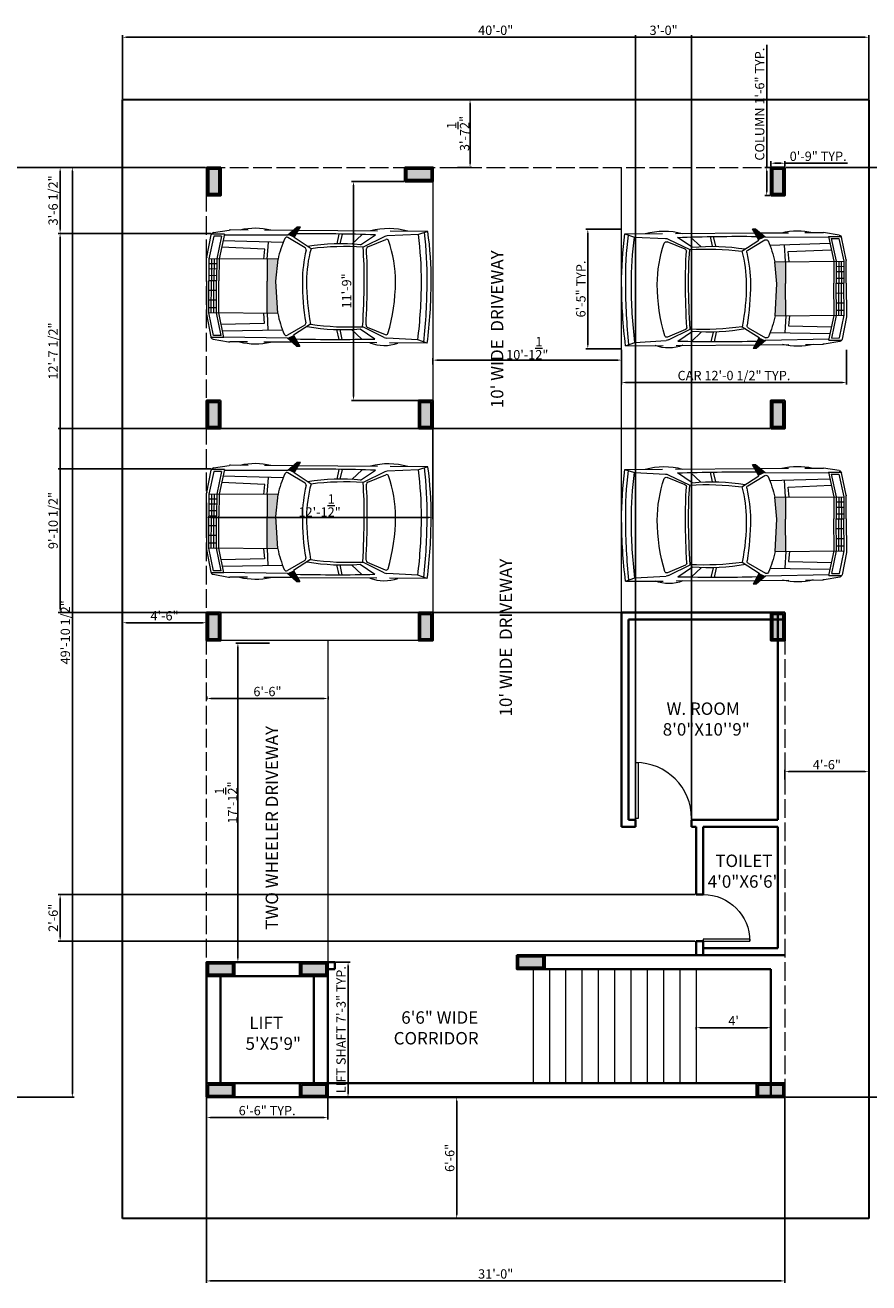
# Model space of a CAD drawing. Units: inches. Extents: x 1678 to 4856, y 4 to 3876.
# Tile 2 of 4: x 2211 to 2753, y 3067 to 3876. Entities that reach past the tile are written whole.
import ezdxf

# ---------------------------------------------------------------- set-up
doc = ezdxf.new("R2010")
doc.units = ezdxf.units.IN
doc.linetypes.add('ACAD_ISO02W100', pattern=[15, 12, -3])
for name, color, linetype, lineweight in [('A-ANNO-TEXT', 7, 'Continuous', 18), ('A-AREA-IDEN', 7, 'Continuous', 18), ('A-FLOR-EVTR', 7, 'Continuous', 35), ('A-FLOR-PRKG', 30, 'Continuous', 18), ('A-WALL-OVHD', 7, 'ACAD_ISO02W100', 18), ('COL', 6, 'Continuous', 40), ('compound wall', 7, 'Continuous', 30), ('DIMENSIONS', 6, 'Continuous', 18), ('doors', 2, 'Continuous', 18), ('FURNITURE', 251, 'Continuous', 5), ('stairs', 1, 'Continuous', 18), ('walls', 7, 'Continuous', 35)]:
    doc.layers.add(name, color=color, linetype=linetype, lineweight=lineweight)
doc.layers.add('CARS', color=150, linetype='Continuous', lineweight=9, true_color=0x386aff)
doc.styles.get("Standard").update_dxf_attribs({"font": 'arial.ttf'})
doc.dimstyles.new('ISO-25', dxfattribs={"dimtxt": 6, "dimasz": 2.5, "dimexe": 1.25, "dimexo": 0.625, "dimtad": 1, "dimdec": 1, "dimlunit": 4, "dimtxsty": 'Standard', "dimcen": 2.5, "dimadec": 0, "dimazin": 0, "dimtfac": 1, "dimtdec": 1, "dimtmove": 0, "dimatfit": 3, "dimfxl": 1, "dimarcsym": 0})

# ---------------------------------------------------------------- blocks, each defined once
blk = doc.blocks.new('*D17')
at = {"layer": 'Defpoints', "color": 0, "transparency": 16777216}
for p in [(2642.23, 3232.03), (2690.23, 3232.03), (2690.23, 3231.08)]:
    blk.add_point(p, dxfattribs=at)
at = {"layer": 'DIMENSIONS', "color": 0, "lineweight": -2, "transparency": 16777216}
for p, q in [((2642.23, 3231.4), (2642.23, 3229.83)), ((2644.73, 3231.08), (2687.73, 3231.08)), ((2690.23, 3231.4), (2690.23, 3229.83))]:
    blk.add_line(p, q, dxfattribs=at)
at = {"layer": 'DIMENSIONS', "color": 0, "transparency": 16777216}
for points in [[(2644.73, 3231.5), (2644.73, 3230.67), (2642.23, 3231.08)], [(2687.73, 3231.5), (2687.73, 3230.67), (2690.23, 3231.08)]]:
    blk.add_solid(points, dxfattribs=at)
at = {"layer": 'DIMENSIONS', "color": 0, "transparency": 16777216, "insert": (2666.23, 3234.71), "char_height": 6, "attachment_point": 5}
blk.add_mtext("4'", dxfattribs=at)
blk = doc.blocks.new('*U2')
for p, q in [((0, 0), (0, -6)), ((40, 0), (40, -6))]:
    blk.add_line(p, q)
blk.add_lwpolyline([(0, 0), (0, 40), (1.75, 40), (1.75, 0)], close=True)
blk.add_arc((0, 0), 40, 0, 90)
blk = doc.blocks.new('car')
at = {"layer": 'FURNITURE'}
for p, q in [((77354.91, -6151.64), (77364.96, -6150.01)), ((77377.06, -6150.02), (77365.73, -6149.95)), ((77405.86, -6150.27), (77387.61, -6150.09)), ((77402.61, -6153), (77408.74, -6147.84)), ((77406.69, -6154.88), (77410.72, -6147.85)), ((77408.74, -6147.84), (77410.72, -6147.85)), ((77460.28, -6150.63), (77409.32, -6150.29)), ((77492.72, -6150.86), (77468.54, -6150.68)), ((77492.72, -6150.86), (77486.64, -6152.92)), ((77350.5, -6167.5), (77353.41, -6153.08)), ((77355.12, -6153.9), (77351.94, -6168.45)), ((77361.89, -6152.63), (77353.6, -6152.58)), ((77360.1, -6153.93), (77355.12, -6153.9)), ((77360.1, -6153.93), (77356.91, -6168.48)), ((77361.89, -6152.63), (77358.42, -6168.49)), ((77399.6, -6158.07), (77360.96, -6156.86)), ((77361.77, -6153.17), (77402.61, -6153)), ((77389.47, -6168.75), (77390.17, -6157.84)), ((77413.78, -6161.37), (77402.69, -6154.78)), ((77417.58, -6162.02), (77406.69, -6154.88)), ((77434.33, -6158.85), (77435.76, -6152.58)), ((77436.36, -6158.86), (77437.79, -6152.61)), ((77450.53, -6152.88), (77443.84, -6159.09)), ((77449.51, -6159.46), (77458.97, -6153.12)), ((77464.99, -6154.22), (77451.07, -6160.93)), ((77454.03, -6160.77), (77465.67, -6156)), ((77486.64, -6152.92), (77466.62, -6153.82)), ((77387.8, -6162.22), (77360.05, -6161.03)), ((77387.14, -6168.73), (77387.8, -6162.22)), ((77350.37, -6182.6), (77350.45, -6167.93)), ((77351.94, -6168.45), (77351.86, -6182.61)), ((77356.87, -6175.06), (77351.9, -6175.03)), ((77356.89, -6171.77), (77351.92, -6171.74)), ((77396.38, -6168.79), (77351.94, -6168.45)), ((77353.59, -6168.46), (77353.52, -6182.62)), ((77355.25, -6168.47), (77355.17, -6182.63)), ((77356.91, -6168.48), (77356.83, -6182.64)), ((77358.42, -6168.49), (77358.34, -6182.65)), ((77389.47, -6168.75), (77389.39, -6182.9)), ((77394.97, -6182.94), (77396.38, -6168.79)), ((77350.37, -6182.6), (77350.29, -6203.77)), ((77351.78, -6203.27), (77351.86, -6182.61)), ((77356.83, -6182.64), (77351.86, -6182.61)), ((77356.85, -6179.35), (77351.88, -6179.32)), ((77353.44, -6203.28), (77353.52, -6182.62)), ((77355.09, -6203.29), (77355.17, -6182.63)), ((77356.75, -6203.3), (77356.83, -6182.64)), ((77358.26, -6203.3), (77358.34, -6182.65)), ((77389.31, -6203.56), (77389.39, -6182.9)), ((77396.22, -6203.6), (77394.97, -6182.94)), ((77356.81, -6188.93), (77351.84, -6188.9)), ((77356.79, -6195.22), (77351.82, -6195.19)), ((77350.33, -6204.2), (77353.07, -6218.65)), ((77396.22, -6203.6), (77351.78, -6203.27)), ((77354.79, -6217.86), (77351.78, -6203.27)), ((77356.77, -6200.01), (77351.8, -6199.98)), ((77359.76, -6217.89), (77356.75, -6203.3)), ((77361.54, -6219.21), (77358.26, -6203.3)), ((77386.98, -6203.55), (77387.56, -6210.07)), ((77389.31, -6203.56), (77389.88, -6214.48)), ((77387.56, -6210.07), (77359.8, -6210.79)), ((77399.31, -6214.36), (77360.66, -6214.97)), ((77413.53, -6211.23), (77402.36, -6217.69)), ((77417.34, -6210.63), (77406.36, -6217.64)), ((77434.05, -6214.07), (77435.4, -6220.37)), ((77436.08, -6214.09), (77437.43, -6220.36)), ((77450.17, -6220.24), (77443.56, -6213.95)), ((77449.23, -6213.65), (77458.62, -6220.1)), ((77464.65, -6219.08), (77450.81, -6212.2)), ((77453.77, -6212.39), (77465.35, -6217.3)), ((77361.54, -6219.21), (77353.24, -6219.16)), ((77354.55, -6220.11), (77364.57, -6221.86)), ((77359.76, -6217.89), (77354.79, -6217.86)), ((77361.43, -6218.67), (77402.26, -6219.46)), ((77376.67, -6222), (77365.35, -6221.93)), ((77405.48, -6222.24), (77387.23, -6222.06)), ((77402.26, -6219.46), (77408.33, -6224.7)), ((77406.36, -6217.64), (77410.3, -6224.72)), ((77459.89, -6222.61), (77408.94, -6222.26)), ((77486.28, -6220.71), (77466.28, -6219.5)), ((77492.34, -6222.84), (77468.16, -6222.66)), ((77492.34, -6222.84), (77486.28, -6220.71)), ((77408.33, -6224.7), (77410.3, -6224.72))]:
    blk.add_line(p, q, dxfattribs=at)
for centre, radius, start, end in [((77365.7, -6154.61), 4.66, 89.65307, 99.2086), ((77381.66, -6191.25), 42.37, 76.12098, 103.18518), ((77467.62, -6193.43), 44.41, 74.13505, 105.34534), ((77264.69, -6182.26), 230.19, 359.66334, 7.84), ((77355.2, -6153.45), 1.83, 99.2086, 168.57498), ((77460.89, -6182.34), 65.93, 155.88538, 168.14022), ((77401.99, -6155.97), 1.38, 59.25451, 155.88538), ((77420.01, -7233.14), 1080.71, 87.93381, 90.63363), ((77436.81, -6291.24), 132.39, 84.49433, 99.30223), ((77466.76, -6157.9), 4.08, 91.9753, 115.73073), ((77466.17, -6157.22), 1.32, 20.32202, 112.28137), ((77393.71, -6182.98), 78.22, 359.66026, 19.58032), ((77269.88, -6182.3), 218.74, 359.66405, 7.71842), ((77223.91, -6182.03), 268.36, 359.66372, 6.50993), ((77502.75, -6183.56), 90.72, 166.83324, 179.67242), ((77413.07, -6162.56), 1.38, 346.15479, 59.25451), ((77496.45, -6183.53), 81.75, 164.74789, 179.67274), ((77440.33, -6345.46), 184.85, 86.67029, 97.06877), ((77169.8, -6181.69), 282.03, 359.66848, 4.22148), ((77454.53, -6161.99), 1.32, 112.28137, 183.63504), ((77132.69, -6181.48), 321.11, 359.66935, 3.46416), ((77352.71, -6167.94), 2.25, 168.57498, 179.65308), ((77569.68, -6183.75), 157.65, 179.74254, 189.48016), ((77553.55, -6183.7), 138.84, 179.73503, 191.18393), ((76982.69, -6181.22), 469.14, 356.21345, 359.74349), ((76906.6, -6180.92), 547.2, 356.8401, 359.74704), ((77352.55, -6182.94), 119.38, 343.64028, 359.75745), ((77167.94, -6182.04), 320.68, 353.07297, 359.72471), ((77104.36, -6181.72), 387.91, 354.0275, 359.72163), ((77164.9, -6182.01), 329.97, 352.89211, 359.72098), ((77352.54, -6203.78), 2.25, 179.65308, 190.73116), ((77460.89, -6190.84), 65.93, 191.16593, 203.42077), ((77412.84, -6210.03), 1.38, 300.05164, 13.15136), ((77438.41, -6081.68), 132.41, 259.88264, 274.68928), ((77442.71, -6027.5), 184.88, 262.11366, 272.51126), ((77454.29, -6211.18), 1.32, 175.6711, 247.02477), ((77354.86, -6218.31), 1.83, 190.73116, 260.09755), ((77365.38, -6217.27), 4.66, 260.09755, 269.65308), ((77381.77, -6180.83), 42.37, 256.12096, 283.18519), ((77401.67, -6216.49), 1.38, 203.42077, 300.05164), ((77434.28, -5139.68), 1080.7, 268.59075, 271.29058), ((77464.57, -6199.01), 25.26, 248.91437, 290.39177), ((77466.47, -6215.42), 4.08, 243.57542, 267.33084), ((77465.87, -6216.09), 1.32, 247.02477, 338.98413)]:
    blk.add_arc(centre, radius, start, end, dxfattribs=at)
for points in [[(77406.69, -6154.88), (77402.61, -6153), (77410.72, -6147.85), (77408.74, -6147.84)], [(77396.22, -6203.6), (77394.97, -6182.94), (77389.31, -6203.56), (77389.47, -6168.75)], [(77394.97, -6182.94), (77396.38, -6168.79), (77389.47, -6168.75)], [(77406.36, -6217.64), (77402.26, -6219.46), (77410.3, -6224.72), (77408.33, -6224.7)]]:
    blk.add_solid(points, dxfattribs=at)
blk = doc.blocks.new('*D23')
at = {"layer": 'Defpoints', "color": 0, "transparency": 16777216}
for p in [(2454.86, 3775.66), (2421.79, 3634.69), (2463.73, 3634.69)]:
    blk.add_point(p, dxfattribs=at)
at = {"layer": 'DIMENSIONS', "color": 0, "lineweight": -2, "transparency": 16777216}
for p, q in [((2454.24, 3775.66), (2420.54, 3775.66)), ((2421.79, 3773.16), (2421.79, 3637.19)), ((2463.1, 3634.69), (2420.54, 3634.69))]:
    blk.add_line(p, q, dxfattribs=at)
at = {"layer": 'DIMENSIONS', "color": 0, "transparency": 16777216}
for points in [[(2421.38, 3773.16), (2422.21, 3773.16), (2421.79, 3775.66)], [(2421.38, 3637.19), (2422.21, 3637.19), (2421.79, 3634.69)]]:
    blk.add_solid(points, dxfattribs=at)
at = {"layer": 'DIMENSIONS', "color": 0, "transparency": 16777216, "insert": (2418.11, 3705.18), "char_height": 6, "attachment_point": 5, "rotation": 90}
blk.add_mtext('11\'-9"', dxfattribs=at)
blk = doc.blocks.new('*D24')
at = {"layer": 'Defpoints', "color": 0, "transparency": 16777216}
for p in [(2472.73, 3616.69), (2327.23, 3569.46), (2472.73, 3559.47)]:
    blk.add_point(p, dxfattribs=at)
at = {"layer": 'DIMENSIONS', "color": 0, "lineweight": -2, "transparency": 16777216}
for p, q in [((2472.73, 3616.07), (2472.73, 3558.22)), ((2327.23, 3568.83), (2327.23, 3558.22)), ((2329.73, 3559.47), (2470.23, 3559.47))]:
    blk.add_line(p, q, dxfattribs=at)
at = {"layer": 'DIMENSIONS', "color": 0, "transparency": 16777216}
for points in [[(2329.73, 3559.89), (2329.73, 3559.06), (2327.23, 3559.47)], [(2470.23, 3559.89), (2470.23, 3559.06), (2472.73, 3559.47)]]:
    blk.add_solid(points, dxfattribs=at)
at = {"layer": 'DIMENSIONS', "color": 0, "transparency": 16777216, "insert": (2399.98, 3567.12), "char_height": 6, "attachment_point": 5}
blk.add_mtext('12\'-1{\\H1x;\\S1/2;}"', dxfattribs=at)
blk = doc.blocks.new('*D25')
at = {"layer": 'Defpoints', "color": 0, "transparency": 16777216}
for p in [(2327.43, 3441.7), (2405.43, 3442.93), (2405.43, 3441.7)]:
    blk.add_point(p, dxfattribs=at)
at = {"layer": 'DIMENSIONS', "color": 0, "lineweight": -2, "transparency": 16777216}
for p, q in [((2327.43, 3442.32), (2327.43, 3444.18)), ((2329.93, 3442.93), (2402.93, 3442.93)), ((2405.43, 3442.32), (2405.43, 3444.18))]:
    blk.add_line(p, q, dxfattribs=at)
at = {"layer": 'DIMENSIONS', "color": 0, "transparency": 16777216}
for points in [[(2329.93, 3443.34), (2329.93, 3442.51), (2327.43, 3442.93)], [(2402.93, 3443.34), (2402.93, 3442.51), (2405.43, 3442.93)]]:
    blk.add_solid(points, dxfattribs=at)
at = {"layer": 'DIMENSIONS', "color": 0, "transparency": 16777216, "insert": (2366.43, 3446.62), "char_height": 6, "attachment_point": 5}
blk.add_mtext('6\'-6"', dxfattribs=at)
blk = doc.blocks.new('*D26')
at = {"layer": 'Defpoints', "color": 0, "transparency": 16777216}
for p in [(2368.46, 3478.61), (2347.41, 3273.28), (2372.98, 3273.28)]:
    blk.add_point(p, dxfattribs=at)
at = {"layer": 'DIMENSIONS', "color": 0, "lineweight": -2, "transparency": 16777216}
for p, q in [((2367.83, 3478.61), (2346.16, 3478.61)), ((2347.41, 3476.11), (2347.41, 3275.78)), ((2372.35, 3273.28), (2346.16, 3273.28))]:
    blk.add_line(p, q, dxfattribs=at)
at = {"layer": 'DIMENSIONS', "color": 0, "transparency": 16777216}
for points in [[(2347, 3476.11), (2347.83, 3476.11), (2347.41, 3478.61)], [(2347, 3275.78), (2347.83, 3275.78), (2347.41, 3273.28)]]:
    blk.add_solid(points, dxfattribs=at)
at = {"layer": 'DIMENSIONS', "color": 0, "transparency": 16777216, "insert": (2339.76, 3375.94), "char_height": 6, "attachment_point": 5, "rotation": 90}
blk.add_mtext('17\'-1{\\H1x;\\S1/2;}"', dxfattribs=at)
blk = doc.blocks.new('*D27')
at = {"layer": 'Defpoints', "color": 0, "transparency": 16777216}
for p in [(2594.23, 3660.65), (2472.86, 3657.11), (2594.23, 3657.11)]:
    blk.add_point(p, dxfattribs=at)
at = {"layer": 'DIMENSIONS', "color": 0, "lineweight": -2, "transparency": 16777216}
for p, q in [((2472.86, 3657.74), (2472.86, 3661.9)), ((2475.36, 3660.65), (2591.73, 3660.65)), ((2594.23, 3657.74), (2594.23, 3661.9))]:
    blk.add_line(p, q, dxfattribs=at)
at = {"layer": 'DIMENSIONS', "color": 0, "transparency": 16777216}
for points in [[(2475.36, 3661.06), (2475.36, 3660.23), (2472.86, 3660.65)], [(2591.73, 3661.06), (2591.73, 3660.23), (2594.23, 3660.65)]]:
    blk.add_solid(points, dxfattribs=at)
at = {"layer": 'DIMENSIONS', "color": 0, "transparency": 16777216, "insert": (2533.55, 3668.35), "char_height": 6, "attachment_point": 5}
blk.add_mtext('10\'-1{\\H1x;\\S1/2;}"', dxfattribs=at)
blk = doc.blocks.new('*D28')
at = {"layer": 'Defpoints', "color": 0, "transparency": 16777216}
for p in [(2493.81, 3186.28), (2488.14, 3108.28), (2493.81, 3108.28)]:
    blk.add_point(p, dxfattribs=at)
at = {"layer": 'DIMENSIONS', "color": 0, "lineweight": -2, "transparency": 16777216}
for p, q in [((2493.18, 3186.28), (2486.89, 3186.28)), ((2488.14, 3183.78), (2488.14, 3110.78)), ((2493.18, 3108.28), (2486.89, 3108.28))]:
    blk.add_line(p, q, dxfattribs=at)
at = {"layer": 'DIMENSIONS', "color": 0, "transparency": 16777216}
for points in [[(2487.72, 3183.78), (2488.55, 3183.78), (2488.14, 3186.28)], [(2487.72, 3110.78), (2488.55, 3110.78), (2488.14, 3108.28)]]:
    blk.add_solid(points, dxfattribs=at)
at = {"layer": 'DIMENSIONS', "color": 0, "transparency": 16777216, "insert": (2484.45, 3147.28), "char_height": 6, "attachment_point": 5, "rotation": 90}
blk.add_mtext('6\'-6"', dxfattribs=at)
blk = doc.blocks.new('*D29')
at = {"layer": 'Defpoints', "color": 0, "transparency": 16777216}
for p in [(2488.14, 3828.28), (2488.14, 3784.66), (2496.74, 3784.66)]:
    blk.add_point(p, dxfattribs=at)
at = {"layer": 'DIMENSIONS', "color": 0, "lineweight": -2, "transparency": 16777216}
for p, q in [((2488.76, 3828.28), (2497.99, 3828.28)), ((2496.74, 3825.78), (2496.74, 3787.16)), ((2488.76, 3784.66), (2497.99, 3784.66))]:
    blk.add_line(p, q, dxfattribs=at)
at = {"layer": 'DIMENSIONS', "color": 0, "transparency": 16777216}
for points in [[(2496.33, 3825.78), (2497.16, 3825.78), (2496.74, 3828.28)], [(2496.33, 3787.16), (2497.16, 3787.16), (2496.74, 3784.66)]]:
    blk.add_solid(points, dxfattribs=at)
at = {"layer": 'DIMENSIONS', "color": 0, "transparency": 16777216, "insert": (2489.04, 3806.47), "char_height": 6, "attachment_point": 5, "rotation": 90}
blk.add_mtext('3\'-7{\\H1x;\\S1/2;}"', dxfattribs=at)
blk = doc.blocks.new('*D30')
at = {"layer": 'Defpoints', "color": 0, "transparency": 16777216}
for p in [(2327.23, 3491.67), (2273.23, 3486.01), (2327.23, 3485.47)]:
    blk.add_point(p, dxfattribs=at)
at = {"layer": 'DIMENSIONS', "color": 0, "lineweight": -2, "transparency": 16777216}
for p, q in [((2273.23, 3486.63), (2273.23, 3492.92)), ((2275.73, 3491.67), (2324.73, 3491.67)), ((2327.23, 3486.1), (2327.23, 3492.92))]:
    blk.add_line(p, q, dxfattribs=at)
at = {"layer": 'DIMENSIONS', "color": 0, "transparency": 16777216}
for points in [[(2275.73, 3492.08), (2275.73, 3491.25), (2273.23, 3491.67)], [(2324.73, 3492.08), (2324.73, 3491.25), (2327.23, 3491.67)]]:
    blk.add_solid(points, dxfattribs=at)
at = {"layer": 'DIMENSIONS', "color": 0, "transparency": 16777216, "insert": (2300.23, 3495.36), "char_height": 6, "attachment_point": 5}
blk.add_mtext('4\'-6"', dxfattribs=at)
blk = doc.blocks.new('*D31')
at = {"layer": 'Defpoints', "color": 0, "transparency": 16777216}
for p in [(2753.23, 3395.85), (2699.23, 3390.15), (2753.23, 3390.15)]:
    blk.add_point(p, dxfattribs=at)
at = {"layer": 'DIMENSIONS', "color": 0, "lineweight": -2, "transparency": 16777216}
for p, q in [((2699.23, 3390.78), (2699.23, 3397.1)), ((2701.73, 3395.85), (2750.73, 3395.85)), ((2753.23, 3390.78), (2753.23, 3397.1))]:
    blk.add_line(p, q, dxfattribs=at)
at = {"layer": 'DIMENSIONS', "color": 0, "transparency": 16777216}
for points in [[(2701.73, 3396.27), (2701.73, 3395.43), (2699.23, 3395.85)], [(2750.73, 3396.27), (2750.73, 3395.43), (2753.23, 3395.85)]]:
    blk.add_solid(points, dxfattribs=at)
at = {"layer": 'DIMENSIONS', "color": 0, "transparency": 16777216, "insert": (2726.23, 3399.54), "char_height": 6, "attachment_point": 5}
blk.add_mtext('4\'-6"', dxfattribs=at)
blk = doc.blocks.new('COLUMN-9x18')
h = blk.add_hatch(color=256)
h.dxf.hatch_style = 1
h.paths.add_polyline_path([(8, 1), (8, 17), (1, 17), (1, 1)])
for points in [[(9, 18), (9, 0), (0, 0), (0, 18)], [(8, 17), (8, 1), (1, 1), (1, 17)]]:
    blk.add_lwpolyline(points, close=True)
blk = doc.blocks.new('SITE-PERIMETER-40x60')
for p, q in [((0, 720), (480, 720)), ((0, 0), (0, 720)), ((480, 720), (480, 0)), ((480, 0), (0, 0))]:
    blk.add_line(p, q)
blk = doc.blocks.new('STAIR-FLIGHT-11-TREAD-LINES')
for p, q in [((0, 73.5), (0, 0)), ((10.5, 73.5), (10.5, 0)), ((21, 73.5), (21, 0)), ((31.5, 73.5), (31.5, 0)), ((42, 73.5), (42, 0)), ((52.5, 73.5), (52.5, 0)), ((63, 73.5), (63, 0)), ((73.5, 73.5), (73.5, 0)), ((84, 73.5), (84, 0)), ((94.5, 73.5), (94.5, 0)), ((105, 73.5), (105, 0))]:
    blk.add_line(p, q)
blk = doc.blocks.new('LIFT-SHAFT-60x69')
for p, q in [((9, 9), (9, 78)), ((69, 9), (9, 9))]:
    blk.add_line(p, q)
blk.add_lwpolyline([(78, 87), (78, 87), (0, 87), (0, 0), (78, 0), (78, 82.5)])
blk.add_lwpolyline([(9, 9), (69, 9), (69, 78), (9, 78)], close=True)
blk = doc.blocks.new('*D40')
at = {"layer": 'Defpoints', "color": 0, "transparency": 16777216}
for p in [(2687.53, 3784.66), (2690.23, 3784.66), (2690.23, 3766.66)]:
    blk.add_point(p, dxfattribs=at)
at = {"layer": 'DIMENSIONS', "color": 0, "lineweight": -2, "transparency": 16777216}
for p, q in [((2687.53, 3784.66), (2687.53, 3863.57)), ((2689.6, 3784.66), (2686.28, 3784.66)), ((2687.53, 3769.16), (2687.53, 3782.16)), ((2689.6, 3766.66), (2686.28, 3766.66))]:
    blk.add_line(p, q, dxfattribs=at)
at = {"layer": 'DIMENSIONS', "color": 0, "transparency": 16777216}
for points in [[(2687.11, 3782.16), (2687.95, 3782.16), (2687.53, 3784.66)], [(2687.11, 3769.16), (2687.95, 3769.16), (2687.53, 3766.66)]]:
    blk.add_solid(points, dxfattribs=at)
at = {"layer": 'DIMENSIONS', "color": 0, "transparency": 16777216, "insert": (2683.8, 3825.37), "char_height": 6, "attachment_point": 5, "rotation": 90}
blk.add_mtext('COLUMN 1\'-6" TYP.', dxfattribs=at)
blk = doc.blocks.new('*D41')
at = {"layer": 'Defpoints', "color": 0, "transparency": 16777216}
for p in [(2690.23, 3784.66), (2699.23, 3787.36), (2699.23, 3784.66)]:
    blk.add_point(p, dxfattribs=at)
at = {"layer": 'DIMENSIONS', "color": 0, "lineweight": -2, "transparency": 16777216}
for p, q in [((2690.23, 3785.29), (2690.23, 3788.61)), ((2699.23, 3785.29), (2699.23, 3788.61)), ((2692.73, 3787.36), (2696.73, 3787.36)), ((2699.23, 3787.36), (2739.55, 3787.36))]:
    blk.add_line(p, q, dxfattribs=at)
at = {"layer": 'DIMENSIONS', "color": 0, "transparency": 16777216}
for points in [[(2692.73, 3787.78), (2692.73, 3786.95), (2690.23, 3787.36)], [(2696.73, 3787.78), (2696.73, 3786.95), (2699.23, 3787.36)]]:
    blk.add_solid(points, dxfattribs=at)
at = {"layer": 'DIMENSIONS', "color": 0, "transparency": 16777216, "insert": (2720.64, 3791.05), "char_height": 6, "attachment_point": 5}
blk.add_mtext('0\'-9" TYP.', dxfattribs=at)
blk = doc.blocks.new('*D42')
at = {"layer": 'Defpoints', "color": 0, "transparency": 16777216}
for p in [(2594.16, 3667.93), (2738.81, 3667.93), (2594.16, 3646.23)]:
    blk.add_point(p, dxfattribs=at)
at = {"layer": 'DIMENSIONS', "color": 0, "lineweight": -2, "transparency": 16777216}
for p, q in [((2594.16, 3667.3), (2594.16, 3644.98)), ((2738.81, 3667.3), (2738.81, 3644.98)), ((2736.31, 3646.23), (2596.66, 3646.23))]:
    blk.add_line(p, q, dxfattribs=at)
at = {"layer": 'DIMENSIONS', "color": 0, "transparency": 16777216}
for points in [[(2596.66, 3646.65), (2596.66, 3645.81), (2594.16, 3646.23)], [(2736.31, 3646.65), (2736.31, 3645.81), (2738.81, 3646.23)]]:
    blk.add_solid(points, dxfattribs=at)
at = {"layer": 'DIMENSIONS', "color": 0, "transparency": 16777216, "insert": (2666.49, 3649.96), "char_height": 6, "attachment_point": 5}
blk.add_mtext('CAR 12\'-0 1/2" TYP.', dxfattribs=at)
blk = doc.blocks.new('*D43')
at = {"layer": 'Defpoints', "color": 0, "transparency": 16777216}
for p in [(2572.47, 3744.93), (2594.16, 3744.93), (2594.16, 3667.93)]:
    blk.add_point(p, dxfattribs=at)
at = {"layer": 'DIMENSIONS', "color": 0, "lineweight": -2, "transparency": 16777216}
for p, q in [((2593.54, 3744.93), (2571.22, 3744.93)), ((2572.47, 3670.43), (2572.47, 3742.43)), ((2593.54, 3667.93), (2571.22, 3667.93))]:
    blk.add_line(p, q, dxfattribs=at)
at = {"layer": 'DIMENSIONS', "color": 0, "transparency": 16777216}
for points in [[(2572.05, 3742.43), (2572.88, 3742.43), (2572.47, 3744.93)], [(2572.05, 3670.43), (2572.88, 3670.43), (2572.47, 3667.93)]]:
    blk.add_solid(points, dxfattribs=at)
at = {"layer": 'DIMENSIONS', "color": 0, "transparency": 16777216, "insert": (2568.78, 3706.43), "char_height": 6, "attachment_point": 5, "rotation": 90}
blk.add_mtext('6\'-5" TYP.', dxfattribs=at)
blk = doc.blocks.new('*D44')
at = {"layer": 'Defpoints', "color": 0, "transparency": 16777216}
for p in [(2405.23, 3273.28), (2418.28, 3273.28), (2405.23, 3186.28)]:
    blk.add_point(p, dxfattribs=at)
at = {"layer": 'DIMENSIONS', "color": 0, "lineweight": -2, "transparency": 16777216}
for p, q in [((2405.85, 3273.28), (2419.53, 3273.28)), ((2418.28, 3188.78), (2418.28, 3270.78)), ((2405.85, 3186.28), (2419.53, 3186.28))]:
    blk.add_line(p, q, dxfattribs=at)
at = {"layer": 'DIMENSIONS', "color": 0, "transparency": 16777216}
for points in [[(2417.86, 3270.78), (2418.7, 3270.78), (2418.28, 3273.28)], [(2417.86, 3188.78), (2418.7, 3188.78), (2418.28, 3186.28)]]:
    blk.add_solid(points, dxfattribs=at)
at = {"layer": 'DIMENSIONS', "color": 0, "transparency": 16777216, "insert": (2414.55, 3229.78), "char_height": 6, "attachment_point": 5, "rotation": 90}
blk.add_mtext('LIFT SHAFT 7\'-3" TYP.', dxfattribs=at)
blk = doc.blocks.new('*D45')
at = {"layer": 'Defpoints', "color": 0, "transparency": 16777216}
for p in [(2327.23, 3186.28), (2405.23, 3186.28), (2405.23, 3173.23)]:
    blk.add_point(p, dxfattribs=at)
at = {"layer": 'DIMENSIONS', "color": 0, "lineweight": -2, "transparency": 16777216}
for p, q in [((2327.23, 3185.65), (2327.23, 3171.98)), ((2405.23, 3185.65), (2405.23, 3171.98)), ((2329.73, 3173.23), (2402.73, 3173.23))]:
    blk.add_line(p, q, dxfattribs=at)
at = {"layer": 'DIMENSIONS', "color": 0, "transparency": 16777216}
for points in [[(2329.73, 3173.64), (2329.73, 3172.81), (2327.23, 3173.23)], [(2402.73, 3173.64), (2402.73, 3172.81), (2405.23, 3173.23)]]:
    blk.add_solid(points, dxfattribs=at)
at = {"layer": 'DIMENSIONS', "color": 0, "transparency": 16777216, "insert": (2366.23, 3176.92), "char_height": 6, "attachment_point": 5}
blk.add_mtext('6\'-6" TYP.', dxfattribs=at)
blk = doc.blocks.new('*D56')
at = {"layer": 'Defpoints', "color": 0, "transparency": 16777216}
for p in [(2146.78, 3784.66), (2240.93, 3784.66), (2146.78, 3186.28)]:
    blk.add_point(p, dxfattribs=at)
at = {"layer": 'DIMENSIONS', "color": 0, "lineweight": -2, "transparency": 16777216}
for p, q in [((2147.41, 3784.66), (2242.18, 3784.66)), ((2240.93, 3188.78), (2240.93, 3782.16)), ((2147.41, 3186.28), (2242.18, 3186.28))]:
    blk.add_line(p, q, dxfattribs=at)
at = {"layer": 'DIMENSIONS', "color": 0, "transparency": 16777216}
for points in [[(2240.52, 3782.16), (2241.35, 3782.16), (2240.93, 3784.66)], [(2240.52, 3188.78), (2241.35, 3188.78), (2240.93, 3186.28)]]:
    blk.add_solid(points, dxfattribs=at)
at = {"layer": 'DIMENSIONS', "color": 0, "transparency": 16777216, "insert": (2237.2, 3485.47), "char_height": 6, "attachment_point": 5, "rotation": 90}
blk.add_mtext('49\'-10 1/2"', dxfattribs=at)
blk = doc.blocks.new('*D57')
at = {"layer": 'Defpoints', "color": 0, "transparency": 16777216}
for p in [(2753.23, 3868.43), (2273.23, 3828.28), (2753.23, 3828.28)]:
    blk.add_point(p, dxfattribs=at)
at = {"layer": 'DIMENSIONS', "color": 0, "lineweight": -2, "transparency": 16777216}
for p, q in [((2273.23, 3828.9), (2273.23, 3869.68)), ((2753.23, 3828.9), (2753.23, 3869.68)), ((2275.73, 3868.43), (2750.73, 3868.43))]:
    blk.add_line(p, q, dxfattribs=at)
at = {"layer": 'DIMENSIONS', "color": 0, "transparency": 16777216}
for points in [[(2275.73, 3868.84), (2275.73, 3868.01), (2273.23, 3868.43)], [(2750.73, 3868.84), (2750.73, 3868.01), (2753.23, 3868.43)]]:
    blk.add_solid(points, dxfattribs=at)
at = {"layer": 'DIMENSIONS', "color": 0, "transparency": 16777216, "insert": (2513.23, 3872.12), "char_height": 6, "attachment_point": 5}
blk.add_mtext('40\'-0"', dxfattribs=at)
blk = doc.blocks.new('*D59')
at = {"layer": 'Defpoints', "color": 0, "transparency": 16777216}
for p in [(2699.23, 3784.66), (2793.38, 3784.66), (2699.23, 3186.28)]:
    blk.add_point(p, dxfattribs=at)
at = {"layer": 'DIMENSIONS', "color": 0, "lineweight": -2, "transparency": 16777216}
for p, q in [((2699.85, 3784.66), (2794.63, 3784.66)), ((2793.38, 3188.78), (2793.38, 3782.16)), ((2699.85, 3186.28), (2794.63, 3186.28))]:
    blk.add_line(p, q, dxfattribs=at)
at = {"layer": 'DIMENSIONS', "color": 0, "transparency": 16777216}
for points in [[(2792.96, 3782.16), (2793.8, 3782.16), (2793.38, 3784.66)], [(2792.96, 3188.78), (2793.8, 3188.78), (2793.38, 3186.28)]]:
    blk.add_solid(points, dxfattribs=at)
at = {"layer": 'DIMENSIONS', "color": 0, "transparency": 16777216, "insert": (2789.65, 3485.47), "char_height": 6, "attachment_point": 5, "rotation": 90}
blk.add_mtext('49\'-10 1/2"', dxfattribs=at)
blk = doc.blocks.new('*D60')
at = {"layer": 'Defpoints', "color": 0, "transparency": 16777216}
for p in [(2327.23, 3186.28), (2699.23, 3186.28), (2699.23, 3068.13)]:
    blk.add_point(p, dxfattribs=at)
at = {"layer": 'DIMENSIONS', "color": 0, "lineweight": -2, "transparency": 16777216}
for p, q in [((2327.23, 3185.65), (2327.23, 3066.88)), ((2699.23, 3185.65), (2699.23, 3066.88)), ((2329.73, 3068.13), (2696.73, 3068.13))]:
    blk.add_line(p, q, dxfattribs=at)
at = {"layer": 'DIMENSIONS', "color": 0, "transparency": 16777216}
for points in [[(2329.73, 3068.54), (2329.73, 3067.71), (2327.23, 3068.13)], [(2696.73, 3068.54), (2696.73, 3067.71), (2699.23, 3068.13)]]:
    blk.add_solid(points, dxfattribs=at)
at = {"layer": 'DIMENSIONS', "color": 0, "transparency": 16777216, "insert": (2513.23, 3071.82), "char_height": 6, "attachment_point": 5}
blk.add_mtext('31\'-0"', dxfattribs=at)
blk = doc.blocks.new('*D74')
at = {"layer": 'Defpoints', "color": 0, "transparency": 16777216}
for p in [(2639.23, 3868.43), (2603.23, 3364.75), (2639.23, 3364.75)]:
    blk.add_point(p, dxfattribs=at)
at = {"layer": 'DIMENSIONS', "color": 0, "lineweight": -2, "transparency": 16777216}
for p, q in [((2603.23, 3365.37), (2603.23, 3869.68)), ((2639.23, 3365.37), (2639.23, 3869.68)), ((2605.73, 3868.43), (2636.73, 3868.43))]:
    blk.add_line(p, q, dxfattribs=at)
at = {"layer": 'DIMENSIONS', "color": 0, "transparency": 16777216}
for points in [[(2605.73, 3868.84), (2605.73, 3868.01), (2603.23, 3868.43)], [(2636.73, 3868.84), (2636.73, 3868.01), (2639.23, 3868.43)]]:
    blk.add_solid(points, dxfattribs=at)
at = {"layer": 'DIMENSIONS', "color": 0, "transparency": 16777216, "insert": (2621.23, 3872.12), "char_height": 6, "attachment_point": 5}
blk.add_mtext('3\'-0"', dxfattribs=at)
blk = doc.blocks.new('*D75')
at = {"layer": 'Defpoints', "color": 0, "transparency": 16777216}
for p in [(2233.08, 3316.78), (2642.23, 3316.78), (2642.23, 3286.78)]:
    blk.add_point(p, dxfattribs=at)
at = {"layer": 'DIMENSIONS', "color": 0, "lineweight": -2, "transparency": 16777216}
for p, q in [((2641.6, 3316.78), (2231.83, 3316.78)), ((2233.08, 3289.28), (2233.08, 3314.28)), ((2641.6, 3286.78), (2231.83, 3286.78))]:
    blk.add_line(p, q, dxfattribs=at)
at = {"layer": 'DIMENSIONS', "color": 0, "transparency": 16777216}
for points in [[(2232.66, 3314.28), (2233.5, 3314.28), (2233.08, 3316.78)], [(2232.66, 3289.28), (2233.5, 3289.28), (2233.08, 3286.78)]]:
    blk.add_solid(points, dxfattribs=at)
at = {"layer": 'DIMENSIONS', "color": 0, "transparency": 16777216, "insert": (2229.39, 3301.78), "char_height": 6, "attachment_point": 5, "rotation": 90}
blk.add_mtext('2\'-6"', dxfattribs=at)
blk = doc.blocks.new('*D82')
at = {"layer": 'Defpoints', "color": 0, "transparency": 16777216}
for p in [(2327.23, 3784.66), (2233.08, 3742.22), (2330.79, 3742.22)]:
    blk.add_point(p, dxfattribs=at)
at = {"layer": 'DIMENSIONS', "color": 0, "lineweight": -2, "transparency": 16777216}
for p, q in [((2326.6, 3784.66), (2231.83, 3784.66)), ((2233.08, 3782.16), (2233.08, 3744.72)), ((2330.17, 3742.22), (2231.83, 3742.22))]:
    blk.add_line(p, q, dxfattribs=at)
at = {"layer": 'DIMENSIONS', "color": 0, "transparency": 16777216}
for points in [[(2232.66, 3782.16), (2233.5, 3782.16), (2233.08, 3784.66)], [(2232.66, 3744.72), (2233.5, 3744.72), (2233.08, 3742.22)]]:
    blk.add_solid(points, dxfattribs=at)
at = {"layer": 'DIMENSIONS', "color": 0, "transparency": 16777216, "insert": (2229.35, 3763.44), "char_height": 6, "attachment_point": 5, "rotation": 90}
blk.add_mtext('3\'-6 1/2"', dxfattribs=at)
blk = doc.blocks.new('*D83')
at = {"layer": 'Defpoints', "color": 0, "transparency": 16777216}
for p in [(2330.79, 3742.22), (2233.08, 3590.79), (2330.81, 3590.79)]:
    blk.add_point(p, dxfattribs=at)
at = {"layer": 'DIMENSIONS', "color": 0, "lineweight": -2, "transparency": 16777216}
for p, q in [((2330.17, 3742.22), (2231.83, 3742.22)), ((2233.08, 3739.72), (2233.08, 3593.29)), ((2330.18, 3590.79), (2231.83, 3590.79))]:
    blk.add_line(p, q, dxfattribs=at)
at = {"layer": 'DIMENSIONS', "color": 0, "transparency": 16777216}
for points in [[(2232.66, 3739.72), (2233.5, 3739.72), (2233.08, 3742.22)], [(2232.66, 3593.29), (2233.5, 3593.29), (2233.08, 3590.79)]]:
    blk.add_solid(points, dxfattribs=at)
at = {"layer": 'DIMENSIONS', "color": 0, "transparency": 16777216, "insert": (2229.35, 3666.5), "char_height": 6, "attachment_point": 5, "rotation": 90}
blk.add_mtext('12\'-7 1/2"', dxfattribs=at)
blk = doc.blocks.new('*D84')
at = {"layer": 'Defpoints', "color": 0, "transparency": 16777216}
for p in [(2690.23, 3616.69), (2233.08, 3498.16), (2690.23, 3498.16)]:
    blk.add_point(p, dxfattribs=at)
at = {"layer": 'DIMENSIONS', "color": 0, "lineweight": -2, "transparency": 16777216}
for p, q in [((2689.6, 3616.69), (2231.83, 3616.69)), ((2233.08, 3614.19), (2233.08, 3500.66)), ((2689.6, 3498.16), (2231.83, 3498.16))]:
    blk.add_line(p, q, dxfattribs=at)
at = {"layer": 'DIMENSIONS', "color": 0, "transparency": 16777216}
for points in [[(2232.66, 3614.19), (2233.5, 3614.19), (2233.08, 3616.69)], [(2232.66, 3500.66), (2233.5, 3500.66), (2233.08, 3498.16)]]:
    blk.add_solid(points, dxfattribs=at)
at = {"layer": 'DIMENSIONS', "color": 0, "transparency": 16777216, "insert": (2229.35, 3557.43), "char_height": 6, "attachment_point": 5, "rotation": 90}
blk.add_mtext('9\'-10 1/2"', dxfattribs=at)

msp = doc.modelspace()

# ---------------------------------------------------------------- linework, layer by layer
at = {"layer": 'A-FLOR-PRKG'}
for p, q in [((2472.86, 3784.66), (2472.86, 3480.16)), ((2594.23, 3498.16), (2594.23, 3784.66)), ((2472.86, 3480.16), (2327.23, 3480.16)), ((2405.23, 3480.16), (2405.23, 3264.28))]:
    msp.add_line(p, q, dxfattribs=at)
at = {"layer": 'A-WALL-OVHD'}
for p, q in [((2327.23, 3784.66), (2699.23, 3784.66)), ((2327.23, 3186.28), (2327.23, 3784.66)), ((2699.23, 3784.66), (2699.23, 3766.66)), ((2699.23, 3498.16), (2699.23, 3186.28)), ((2699.23, 3186.28), (2327.23, 3186.28))]:
    msp.add_line(p, q, dxfattribs=at)
at = {"layer": 'walls'}
for p, q in [((2594.23, 3498.16), (2594.23, 3360.28)), ((2690.23, 3498.16), (2594.23, 3498.16)), ((2699.23, 3498.16), (2646.73, 3498.16)), ((2694.73, 3497.16), (2694.73, 3364.75)), ((2699.23, 3493.66), (2598.73, 3493.66)), ((2598.73, 3493.66), (2598.73, 3364.75)), ((2594.23, 3360.28), (2603.23, 3360.28)), ((2598.73, 3364.75), (2603.23, 3364.75)), ((2603.23, 3364.75), (2603.23, 3360.28)), ((2639.23, 3364.75), (2639.23, 3360.28)), ((2639.23, 3364.75), (2694.73, 3364.75)), ((2639.23, 3360.28), (2642.23, 3360.28)), ((2642.23, 3360.28), (2642.23, 3316.78)), ((2646.73, 3360.28), (2646.73, 3316.78)), ((2646.73, 3360.28), (2694.73, 3360.28)), ((2694.73, 3360.28), (2694.73, 3282.28)), ((2646.73, 3316.78), (2642.23, 3316.78)), ((2646.73, 3286.78), (2642.23, 3286.78)), ((2642.23, 3286.78), (2642.23, 3277.78)), ((2646.73, 3286.78), (2646.73, 3277.78)), ((2646.73, 3282.28), (2694.73, 3282.28)), ((2409.73, 3273.28), (2336.23, 3273.28)), ((2409.73, 3273.28), (2409.73, 3268.78)), ((2409.73, 3273.28), (2409.73, 3268.78)), ((2544.78, 3277.78), (2699.23, 3277.78)), ((2409.73, 3268.78), (2405.23, 3268.78)), ((2690.23, 3268.78), (2526.78, 3268.78)), ((2690.23, 3268.78), (2690.23, 3186.28)), ((2405.23, 3195.28), (2690.04, 3195.28)), ((2699.23, 3186.28), (2327.23, 3186.28))]:
    msp.add_line(p, q, dxfattribs=at)

# ---------------------------------------------------------------- block references
at = {"layer": 'A-FLOR-EVTR'}
msp.add_blockref('LIFT-SHAFT-60x69', (2327.23, 3186.28), dxfattribs=at)
at = {"layer": 'CARS'}
for p in [(-75023.14, 9894.35), (-75023.13, 9742.92)]:
    msp.add_blockref('car', p, dxfattribs=at)
at = {"layer": 'CARS', "xscale": -1}
for p in [(80089.1, 9892.76), (80089.1, 9741.16)]:
    msp.add_blockref('car', p, dxfattribs=at)
at = {"layer": 'COL'}
for p in [(2327.47, 3766.66), (2690.23, 3766.66), (2327.23, 3616.66), (2463.73, 3616.69), (2690.23, 3616.69), (2327.23, 3480.16), (2463.73, 3480.16), (2690.23, 3480.16)]:
    msp.add_blockref('COLUMN-9x18', p, dxfattribs=at)
for p, rotation in [((2472.86, 3775.66), 90.0000000000118), ((2345.23, 3264.28), 90.00000000000551), ((2405.23, 3264.28), 90.00000000000551), ((2544.78, 3268.78), 90.0000000000076), ((2345.23, 3186.28), 90.00000000000551), ((2405.23, 3186.28), 90.00000000000551), ((2699.04, 3186.28), 90.0000000000076)]:
    msp.add_blockref('COLUMN-9x18', p, dxfattribs=dict(at, rotation=rotation))
at = {"layer": 'compound wall', "rotation": 180}
msp.add_blockref('SITE-PERIMETER-40x60', (2753.23, 3828.28), dxfattribs=at)
at = {"layer": 'doors', "xscale": 0.9, "yscale": 0.9, "zscale": 0.9}
msp.add_blockref('*U2', (2603.23, 3365.68), dxfattribs=at)
at = {"layer": 'doors', "xscale": -0.75, "yscale": 0.75, "zscale": 0.75, "rotation": 270}
msp.add_blockref('*U2', (2646.73, 3286.78), dxfattribs=at)
at = {"layer": 'stairs'}
msp.add_blockref('STAIR-FLIGHT-11-TREAD-LINES', (2537.23, 3195.28), dxfattribs=at)

# ---------------------------------------------------------------- texts
at = {"layer": 'A-ANNO-TEXT', "char_height": 8, "attachment_point": 1, "rotation": 90}
for s, insert in [("10' WIDE  DRIVEWAY", (2510.13, 3629.73)), ("10' WIDE  DRIVEWAY", (2515.7, 3431.35)), ('TWO WHEELER DRIVEWAY', (2365.27, 3294.09))]:
    msp.add_mtext_dynamic_manual_height_columns(s, width=187.9722, gutter_width=12.5, heights=[0], dxfattribs=dict(at, insert=insert))
at = {"layer": 'A-AREA-IDEN', "char_height": 8, "attachment_point": 1}
for s, insert in [(' W. ROOM\\P8\'0"X10\'\'9"', (2620.67, 3440.36)), ('  TOILET\\P4\'0"X6\'6"', (2649.6, 3342.47)), (' LIFT\\P5\'X5\'9"', (2352.33, 3238.17)), ('  6\'6" WIDE\\PCORRIDOR', (2447.61, 3241.61))]:
    msp.add_mtext_dynamic_manual_height_columns(s, width=58.5808, gutter_width=12.5, heights=[0], dxfattribs=dict(at, insert=insert))

# ---------------------------------------------------------------- dimensions: what is measured, and where the dimension line sits
at = {"layer": 'DIMENSIONS'}
for base, p1, p2, override, picture, middle in [((2753.23, 3868.43), (2273.23, 3828.28), (2753.23, 3828.28), {"dimdec": 1, "dimlfac": 1, "dimrnd": 0, "dimzin": 1, "dimdsep": 46, "dimlunit": 4, "dimfrac": 2}, '*D57', (2513.23, 3872.12)), ((2639.23, 3868.43), (2603.23, 3364.75), (2639.23, 3364.75), {"dimdec": 1, "dimlfac": 1, "dimrnd": 0, "dimzin": 1, "dimdsep": 46, "dimlunit": 4, "dimfrac": 2}, '*D74', (2621.23, 3872.12)), ((2594.23, 3660.65), (2472.86, 3657.11), (2594.23, 3657.11), {"dimclrd": 0, "dimclre": 0, "dimclrt": 0}, '*D27', (2533.55, 3668.35)), ((2472.73, 3559.47), (2327.23, 3569.46), (2472.73, 3616.69), {"dimclrd": 0, "dimclre": 0, "dimclrt": 0}, '*D24', (2399.98, 3567.12)), ((2327.23, 3491.67), (2273.23, 3486.01), (2327.23, 3485.47), {"dimclrd": 0, "dimclre": 0, "dimclrt": 0}, '*D30', (2300.23, 3495.36)), ((2405.43, 3442.93), (2327.43, 3441.7), (2405.43, 3441.7), {"dimclrd": 0, "dimclre": 0, "dimclrt": 0}, '*D25', (2366.43, 3446.62)), ((2753.23, 3395.85), (2699.23, 3390.15), (2753.23, 3390.15), {"dimclrd": 0, "dimclre": 0, "dimclrt": 0}, '*D31', (2726.23, 3399.54)), ((2690.23, 3231.08), (2642.23, 3232.03), (2690.23, 3232.03), {"dimclrd": 0, "dimclre": 0, "dimclrt": 0}, '*D17', (2666.23, 3234.71)), ((2699.23, 3068.13), (2327.23, 3186.28), (2699.23, 3186.28), {"dimdec": 1, "dimlfac": 1, "dimrnd": 0, "dimzin": 1, "dimdsep": 46, "dimlunit": 4, "dimfrac": 2}, '*D60', (2513.23, 3071.82))]:
    dim = msp.add_linear_dim(base=base, p1=p1, p2=p2, dimstyle='ISO-25', override=override, dxfattribs=at)
    dim.commit()
    dim.dimension.update_dxf_attribs({"geometry": picture, "text_midpoint": middle})
for base, p1, p2, angle, text, picture, middle in [((2687.53, 3784.66), (2690.23, 3766.66), (2690.23, 3784.66), 90, 'COLUMN <> TYP.', '*D40', (2683.8, 3825.37)), ((2572.47, 3744.93), (2594.16, 3667.93), (2594.16, 3744.93), 90, '<> TYP.', '*D43', (2568.78, 3706.43)), ((2594.1642, 3646.2314), (2738.81, 3667.9282), (2594.1642, 3667.9282), 180, 'CAR <> TYP.', '*D42', (2666.4871, 3649.9587)), ((2418.28, 3273.28), (2405.23, 3186.28), (2405.23, 3273.28), 90, 'LIFT SHAFT <> TYP.', '*D44', (2414.55, 3229.78))]:
    dim = msp.add_linear_dim(base=base, p1=p1, p2=p2, angle=angle, text=text, dimstyle='ISO-25', override={"dimdec": 1, "dimlfac": 1, "dimrnd": 0, "dimzin": 1, "dimdsep": 46, "dimlunit": 4, "dimfrac": 2}, dxfattribs=at)
    dim.commit()
    dim.dimension.update_dxf_attribs({"geometry": picture, "text_midpoint": middle})
for base, p1, p2, override, picture, middle in [((2496.74, 3784.66), (2488.14, 3828.28), (2488.14, 3784.66), {"dimclrd": 0, "dimclre": 0, "dimclrt": 0}, '*D29', (2489.04, 3806.47)), ((2240.93, 3784.66), (2146.78, 3186.28), (2146.78, 3784.66), {"dimdec": 1, "dimlfac": 1, "dimrnd": 0, "dimzin": 1, "dimdsep": 46, "dimlunit": 4, "dimfrac": 2}, '*D56', (2237.2, 3485.47)), ((2233.08, 3742.22), (2327.23, 3784.66), (2330.79, 3742.22), {"dimdec": 1, "dimlfac": 1, "dimrnd": 0, "dimzin": 1, "dimdsep": 46, "dimlunit": 4, "dimfrac": 2}, '*D82', (2229.35, 3763.44)), ((2793.38, 3784.66), (2699.23, 3186.28), (2699.23, 3784.66), {"dimdec": 1, "dimlfac": 1, "dimrnd": 0, "dimzin": 1, "dimdsep": 46, "dimlunit": 4, "dimfrac": 2}, '*D59', (2789.65, 3485.47)), ((2421.79, 3634.69), (2454.86, 3775.66), (2463.73, 3634.69), {"dimclrd": 0, "dimclre": 0, "dimclrt": 0}, '*D23', (2418.11, 3705.18)), ((2233.08, 3590.79), (2330.79, 3742.22), (2330.81, 3590.79), {"dimdec": 1, "dimlfac": 1, "dimrnd": 0, "dimzin": 1, "dimdsep": 46, "dimlunit": 4, "dimfrac": 2}, '*D83', (2229.35, 3666.5)), ((2233.08, 3498.16), (2690.23, 3616.69), (2690.23, 3498.16), {"dimdec": 1, "dimlfac": 1, "dimrnd": 0, "dimzin": 1, "dimdsep": 46, "dimlunit": 4, "dimfrac": 2}, '*D84', (2229.35, 3557.43)), ((2347.41, 3273.28), (2368.46, 3478.61), (2372.98, 3273.28), {"dimclrd": 0, "dimclre": 0, "dimclrt": 0}, '*D26', (2339.76, 3375.94)), ((2233.08, 3316.78), (2642.23, 3286.78), (2642.23, 3316.78), {"dimdec": 1, "dimlfac": 1, "dimrnd": 0, "dimzin": 1, "dimdsep": 46, "dimlunit": 4, "dimfrac": 2}, '*D75', (2229.39, 3301.78)), ((2488.14, 3108.28), (2493.81, 3186.28), (2493.81, 3108.28), {"dimclrd": 0, "dimclre": 0, "dimclrt": 0}, '*D28', (2484.45, 3147.28))]:
    dim = msp.add_linear_dim(base=base, p1=p1, p2=p2, angle=90, dimstyle='ISO-25', override=override, dxfattribs=at)
    dim.commit()
    dim.dimension.update_dxf_attribs({"geometry": picture, "text_midpoint": middle})
for base, p1, p2, picture, middle in [((2699.23, 3787.36), (2690.23, 3784.66), (2699.23, 3784.66), '*D41', (2720.64, 3791.05)), ((2405.23, 3173.23), (2327.23, 3186.28), (2405.23, 3186.28), '*D45', (2366.23, 3176.92))]:
    dim = msp.add_linear_dim(base=base, p1=p1, p2=p2, text='<> TYP.', dimstyle='ISO-25', override={"dimdec": 1, "dimlfac": 1, "dimrnd": 0, "dimzin": 1, "dimdsep": 46, "dimlunit": 4, "dimfrac": 2}, dxfattribs=at)
    dim.commit()
    dim.dimension.update_dxf_attribs({"geometry": picture, "text_midpoint": middle})

doc.saveas('drawing.dxf')
